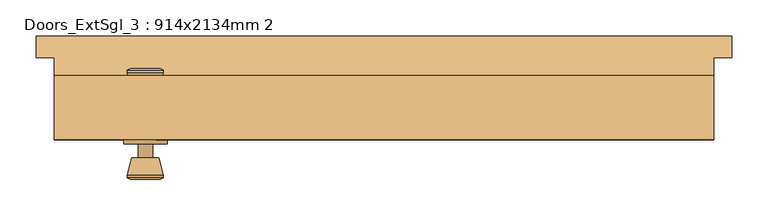
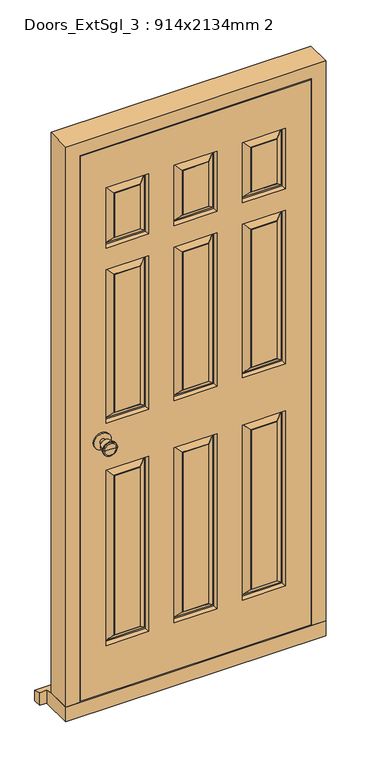
"""IFC4 building model written with IfcOpenShell, lengths in millimetres: door geometry, Doors_ExtSgl_3 : 914x2134mm 2."""

from ifc_helpers import new_model, si_unit, point, frame, frame_2d, origin, place, context, project, spatial, polyline, circle_curve, trimmed, segment, composite_curve, outline, extrude, faceted_brep, source, transform, mapped, element, save
from ifc_brep_helpers import plane_surface, cylinder_surface, revolved_surface, advanced_brep


def doors_extsgl_3_914x2134mm_2_3fd9b232(model_context):
    return source(origin(), model_context, "Body", "SolidModel", [
        advanced_brep(
        [(-330.6666667, -43.8, 1000.0), (-320.6666667, -43.8, 1000.0), (-340.6666667, -43.8, 1000.0), (-310.1907991, -92.8, 1000.0), (-330.6666667, -92.8, 1000.0), (-351.1425342, -92.8, 1000.0), (-305.6666667, -90.9721319, 1000.0), (-355.6666667, -90.9721319, 1000.0), (-305.6666667, -87.5084537, 1000.0), (-355.6666667, -87.5084537, 1000.0), (-312.0304306, -62.8, 1000.0), (-349.3029027, -62.8, 1000.0), (-320.6666667, -62.8, 1000.0), (-340.6666667, -62.8, 1000.0)],
        [
            (0, 1),
            (1, 2, circle_curve(frame((-330.6666667, -43.8, 1000.0), z_axis=(0.0, 1.0, 0.0), x_axis=(-1.0, 0.0, 0.0)), 10.0)),
            (2, 0),
            (2, 1, circle_curve(frame((-330.6666667, -43.8, 1000.0), z_axis=(0.0, 1.0, 0.0), x_axis=(-1.0, 0.0, 0.0)), 10.0)),
            (3, 4),
            (4, 5),
            (5, 3, circle_curve(frame((-330.6666667, -92.8, 1000.0), z_axis=(0.0, -1.0, 0.0), x_axis=(-1.0, 0.0, 0.0)), 20.4758676)),
            (3, 5, circle_curve(frame((-330.6666667, -92.8, 1000.0), z_axis=(0.0, -1.0, 0.0), x_axis=(-1.0, 0.0, 0.0)), 20.4758676)),
            (6, 3),
            (5, 7),
            (7, 6, circle_curve(frame((-330.6666667, -90.9721319, 1000.0), z_axis=(0.0, -1.0, 0.0), x_axis=(-1.0, 0.0, 0.0)), 25.0)),
            (6, 7, circle_curve(frame((-330.6666667, -90.9721319, 1000.0), z_axis=(0.0, -1.0, 0.0), x_axis=(-1.0, 0.0, 0.0)), 25.0)),
            (8, 6),
            (7, 9),
            (9, 8, circle_curve(frame((-330.6666667, -87.5084537, 1000.0), z_axis=(0.0, -1.0, 0.0), x_axis=(-1.0, 0.0, 0.0)), 25.0)),
            (8, 9, circle_curve(frame((-330.6666667, -87.5084537, 1000.0), z_axis=(0.0, -1.0, 0.0), x_axis=(-1.0, 0.0, 0.0)), 25.0)),
            (10, 8),
            (9, 11),
            (11, 10, circle_curve(frame((-330.6666667, -62.8, 1000.0), z_axis=(0.0, -1.0, 0.0), x_axis=(-1.0, 0.0, 0.0)), 18.636236)),
            (10, 11, circle_curve(frame((-330.6666667, -62.8, 1000.0), z_axis=(0.0, -1.0, 0.0), x_axis=(-1.0, 0.0, 0.0)), 18.636236)),
            (12, 10),
            (11, 13),
            (13, 12, circle_curve(frame((-330.6666667, -62.8, 1000.0), z_axis=(0.0, -1.0, 0.0), x_axis=(-1.0, 0.0, 0.0)), 10.0)),
            (12, 13, circle_curve(frame((-330.6666667, -62.8, 1000.0), z_axis=(0.0, -1.0, 0.0), x_axis=(-1.0, 0.0, 0.0)), 10.0)),
            (1, 12),
            (13, 2),
        ],
        [
            plane_surface(frame((-330.6666667, -43.8, 1000.0), z_axis=(0.0, 1.0, 0.0), x_axis=(-1.0, 0.0, 0.0))),
            plane_surface(frame((-330.6666667, -92.8, 1000.0), z_axis=(0.0, -1.0, 0.0), x_axis=(-1.0, 0.0, 0.0))),
            revolved_surface(polyline([(-351.1425342, -92.8, 1000.0), (-355.6666667, -90.9721319, 1000.0)]), (-330.6666667, -43.8, 1000.0), (0.0, 1.0, 0.0)),
            cylinder_surface(frame((-330.6666667, -43.8, 1000.0), z_axis=(0.0, 1.0, 0.0), x_axis=(-1.0, 0.0, 0.0)), 25.0),
            revolved_surface(polyline([(-355.6666667, -87.5084537, 1000.0), (-349.3029027, -62.8, 1000.0)]), (-330.6666667, -43.8, 1000.0), (0.0, 1.0, 0.0)),
            plane_surface(frame((-330.6666667, -62.8, 1000.0), z_axis=(0.0, 1.0, 0.0), x_axis=(-1.0, 0.0, 0.0))),
            cylinder_surface(frame((-330.6666667, -43.8, 1000.0), z_axis=(0.0, 1.0, 0.0), x_axis=(-1.0, 0.0, 0.0)), 10.0),
        ],
        [
            (0, [[1, 2, 3]]),
            (0, [[-3, 4, -1]]),
            (1, [[5, 6, 7]]),
            (1, [[-6, -5, 8]]),
            (2, [[9, -7, 10, 11]]),
            (2, [[-10, -8, -9, 12]]),
            (3, [[13, -11, 14, 15]]),
            (3, [[-14, -12, -13, 16]]),
            (4, [[17, -15, 18, 19]]),
            (4, [[-18, -16, -17, 20]]),
            (5, [[21, -19, 22, 23]]),
            (5, [[-22, -20, -21, 24]]),
            (6, [[25, -23, 26, -2]]),
            (6, [[-26, -24, -25, -4]]),
        ],
    ),
        extrude(outline(composite_curve([segment(trimmed(circle_curve(frame_2d((1000.0, -330.6666667)), 30.0), [point((1000.0, -360.6666667))], [point((1000.0, -300.6666667))], False, "CARTESIAN"), True, "CONTINUOUS"), segment(trimmed(circle_curve(frame_2d((1000.0, -330.6666667)), 30.0), [point((1000.0, -300.6666667))], [point((1000.0, -360.6666667))], False, "CARTESIAN"), True, "CONTINUOUS")], self_intersect=False)), frame((0.0, -43.8, 0.0), z_axis=(0.0, 1.0, 0.0), x_axis=(0.0, 0.0, 1.0)), (0.0, 0.0, 1.0), 6.0),
        advanced_brep(
        [(-330.6666667, 12.2, 1000.0), (-340.6666667, 12.2, 1000.0), (-320.6666667, 12.2, 1000.0), (-310.1907991, 61.2, 1000.0), (-351.1425342, 61.2, 1000.0), (-330.6666667, 61.2, 1000.0), (-305.6666667, 59.3721319, 1000.0), (-355.6666667, 59.3721319, 1000.0), (-305.6666667, 55.9084537, 1000.0), (-355.6666667, 55.9084537, 1000.0), (-312.0304306, 31.2, 1000.0), (-349.3029027, 31.2, 1000.0), (-320.6666667, 31.2, 1000.0), (-340.6666667, 31.2, 1000.0)],
        [
            (0, 1),
            (1, 2, circle_curve(frame((-330.6666667, 12.2, 1000.0), z_axis=(0.0, -1.0, 0.0), x_axis=(-1.0, 0.0, 0.0)), 10.0)),
            (2, 0),
            (2, 1, circle_curve(frame((-330.6666667, 12.2, 1000.0), z_axis=(0.0, -1.0, 0.0), x_axis=(-1.0, 0.0, 0.0)), 10.0)),
            (3, 4, circle_curve(frame((-330.6666667, 61.2, 1000.0), z_axis=(0.0, 1.0, 0.0), x_axis=(-1.0, 0.0, 0.0)), 20.4758676)),
            (4, 5),
            (5, 3),
            (4, 3, circle_curve(frame((-330.6666667, 61.2, 1000.0), z_axis=(0.0, 1.0, 0.0), x_axis=(-1.0, 0.0, 0.0)), 20.4758676)),
            (6, 7, circle_curve(frame((-330.6666667, 59.3721319, 1000.0), z_axis=(0.0, 1.0, 0.0), x_axis=(-1.0, 0.0, 0.0)), 25.0)),
            (7, 4),
            (3, 6),
            (7, 6, circle_curve(frame((-330.6666667, 59.3721319, 1000.0), z_axis=(0.0, 1.0, 0.0), x_axis=(-1.0, 0.0, 0.0)), 25.0)),
            (8, 9, circle_curve(frame((-330.6666667, 55.9084537, 1000.0), z_axis=(0.0, 1.0, 0.0), x_axis=(-1.0, 0.0, 0.0)), 25.0)),
            (9, 7),
            (6, 8),
            (9, 8, circle_curve(frame((-330.6666667, 55.9084537, 1000.0), z_axis=(0.0, 1.0, 0.0), x_axis=(-1.0, 0.0, 0.0)), 25.0)),
            (10, 11, circle_curve(frame((-330.6666667, 31.2, 1000.0), z_axis=(0.0, 1.0, 0.0), x_axis=(-1.0, 0.0, 0.0)), 18.636236)),
            (11, 9),
            (8, 10),
            (11, 10, circle_curve(frame((-330.6666667, 31.2, 1000.0), z_axis=(0.0, 1.0, 0.0), x_axis=(-1.0, 0.0, 0.0)), 18.636236)),
            (12, 13, circle_curve(frame((-330.6666667, 31.2, 1000.0), z_axis=(0.0, 1.0, 0.0), x_axis=(-1.0, 0.0, 0.0)), 10.0)),
            (13, 11),
            (10, 12),
            (13, 12, circle_curve(frame((-330.6666667, 31.2, 1000.0), z_axis=(0.0, 1.0, 0.0), x_axis=(-1.0, 0.0, 0.0)), 10.0)),
            (1, 13),
            (12, 2),
        ],
        [
            plane_surface(frame((-330.6666667, 12.2, 1000.0), z_axis=(0.0, -1.0, 0.0), x_axis=(-1.0, 0.0, 0.0))),
            plane_surface(frame((-330.6666667, 61.2, 1000.0), z_axis=(0.0, 1.0, 0.0), x_axis=(-1.0, 0.0, 0.0))),
            revolved_surface(polyline([(-351.1425342, 61.2, 1000.0), (-355.6666667, 59.3721319, 1000.0)]), (-330.6666667, 12.2, 1000.0), (0.0, -1.0, 0.0)),
            cylinder_surface(frame((-330.6666667, 12.2, 1000.0), z_axis=(0.0, -1.0, 0.0), x_axis=(-1.0, 0.0, 0.0)), 25.0),
            revolved_surface(polyline([(-355.6666667, 55.9084537, 1000.0), (-349.3029027, 31.2, 1000.0)]), (-330.6666667, 12.2, 1000.0), (0.0, -1.0, 0.0)),
            plane_surface(frame((-330.6666667, 31.2, 1000.0), z_axis=(0.0, -1.0, 0.0), x_axis=(-1.0, 0.0, 0.0))),
            cylinder_surface(frame((-330.6666667, 12.2, 1000.0), z_axis=(0.0, -1.0, 0.0), x_axis=(-1.0, 0.0, 0.0)), 10.0),
        ],
        [
            (0, [[1, 2, 3]]),
            (0, [[-3, 4, -1]]),
            (1, [[5, 6, 7]]),
            (1, [[8, -7, -6]]),
            (2, [[9, 10, -5, 11]]),
            (2, [[12, -11, -8, -10]]),
            (3, [[13, 14, -9, 15]]),
            (3, [[16, -15, -12, -14]]),
            (4, [[17, 18, -13, 19]]),
            (4, [[20, -19, -16, -18]]),
            (5, [[21, 22, -17, 23]]),
            (5, [[24, -23, -20, -22]]),
            (6, [[-2, 25, -21, 26]]),
            (6, [[-4, -26, -24, -25]]),
        ],
    ),
        extrude(outline(composite_curve([segment(trimmed(circle_curve(frame_2d((1000.0, -330.6666667)), 30.0), [point((1000.0, -360.6666667))], [point((1000.0, -300.6666667))], False, "CARTESIAN"), True, "CONTINUOUS"), segment(trimmed(circle_curve(frame_2d((1000.0, -330.6666667)), 30.0), [point((1000.0, -300.6666667))], [point((1000.0, -360.6666667))], False, "CARTESIAN"), True, "CONTINUOUS")], self_intersect=False)), frame((0.0, 6.2, 0.0), z_axis=(0.0, 1.0, 0.0), x_axis=(0.0, 0.0, 1.0)), (0.0, 0.0, 1.0), 6.0),
        faceted_brep([(386.7333333, 51.2, 54.5), (457.2333333, 51.2, 54.5), (457.2333333, -37.8, 54.5), (408.7333333, -37.8, 54.5), (408.7333333, 9.2, 54.5), (386.7333333, 9.2, 54.5), (386.7333333, 51.2, 2063.1), (-386.6666667, 51.2, 2063.1), (-386.6666667, 51.2, 54.5), (-457.1666667, 51.2, 54.5), (-457.1666667, 51.2, 2133.6), (457.2333333, 51.2, 2133.6), (457.2333333, -37.8, 2133.6), (-457.1666667, -37.8, 2133.6), (-457.1666667, -37.8, 54.5), (-408.6666667, -37.8, 54.5), (-408.6666667, -37.8, 2085.1), (408.7333333, -37.8, 2085.1), (408.7333333, 9.2, 2085.1), (-408.6666667, 9.2, 2085.1), (-408.6666667, 9.2, 54.5), (-386.6666667, 9.2, 54.5), (-386.6666667, 9.2, 2063.1), (386.7333333, 9.2, 2063.1)], [[[0, 1, 2, 3, 4, 5]], [[1, 0, 6, 7, 8, 9, 10, 11]], [[2, 1, 11, 12]], [[3, 2, 12, 13, 14, 15, 16, 17]], [[4, 3, 17, 18]], [[5, 4, 18, 19, 20, 21, 22, 23]], [[0, 5, 23, 6]], [[8, 7, 22, 21]], [[9, 8, 21, 20, 15, 14]], [[10, 9, 14, 13]], [[16, 15, 20, 19]], [[11, 10, 13, 12]], [[17, 16, 19, 18]], [[7, 6, 23, 22]]]),
        faceted_brep([(405.7333333, -37.8, 58.5), (405.7333333, -37.8, 2082.1), (-406.5916961, -37.8, 2082.1), (-406.5916961, -37.8, 58.5), (-165.2, -37.8, 883.5), (-165.2, -37.8, 233.5), (-315.6666667, -37.8, 233.5), (-315.6666667, -37.8, 883.5), (315.7333333, -37.8, 883.5), (315.7333333, -37.8, 233.5), (165.2666667, -37.8, 233.5), (165.2666667, -37.8, 883.5), (75.2666667, -37.8, 883.5), (75.2666667, -37.8, 233.5), (-75.2, -37.8, 233.5), (-75.2, -37.8, 883.5), (-315.6666667, -37.8, 1058.5), (-315.6666667, -37.8, 1628.5), (-165.2, -37.8, 1628.5), (-165.2, -37.8, 1058.5), (75.2666667, -37.8, 1628.5), (75.2666667, -37.8, 1058.5), (-75.2, -37.8, 1058.5), (-75.2, -37.8, 1628.5), (315.7333333, -37.8, 1628.5), (315.7333333, -37.8, 1058.5), (165.2666667, -37.8, 1058.5), (165.2666667, -37.8, 1628.5), (-165.2, -37.8, 1932.1), (-165.2, -37.8, 1708.5), (-315.6666667, -37.8, 1708.5), (-315.6666667, -37.8, 1932.1), (75.2666667, -37.8, 1932.1), (75.2666667, -37.8, 1708.5), (-75.2, -37.8, 1708.5), (-75.2, -37.8, 1932.1), (315.7333333, -37.8, 1932.1), (315.7333333, -37.8, 1708.5), (165.2666667, -37.8, 1708.5), (165.2666667, -37.8, 1932.1), (-195.2, -37.8, 263.5), (-195.2, -37.8, 853.5), (-285.6666667, -37.8, 853.5), (-285.6666667, -37.8, 263.5), (285.7333333, -37.8, 263.5), (285.7333333, -37.8, 853.5), (195.2666667, -37.8, 853.5), (195.2666667, -37.8, 263.5), (45.2666667, -37.8, 263.5), (45.2666667, -37.8, 853.5), (-45.2, -37.8, 853.5), (-45.2, -37.8, 263.5), (-285.6666667, -37.8, 1598.5), (-285.6666667, -37.8, 1088.5), (-195.2, -37.8, 1088.5), (-195.2, -37.8, 1598.5), (45.2666667, -37.8, 1088.5), (45.2666667, -37.8, 1598.5), (-45.2, -37.8, 1598.5), (-45.2, -37.8, 1088.5), (285.7333333, -37.8, 1088.5), (285.7333333, -37.8, 1598.5), (195.2666667, -37.8, 1598.5), (195.2666667, -37.8, 1088.5), (-195.2, -37.8, 1738.5), (-195.2, -37.8, 1902.1), (-285.6666667, -37.8, 1902.1), (-285.6666667, -37.8, 1738.5), (45.2666667, -37.8, 1738.5), (45.2666667, -37.8, 1902.1), (-45.2, -37.8, 1902.1), (-45.2, -37.8, 1738.5), (285.7333333, -37.8, 1738.5), (285.7333333, -37.8, 1902.1), (195.2666667, -37.8, 1902.1), (195.2666667, -37.8, 1738.5), (405.7333333, 6.2, 58.5), (-406.5916961, 6.2, 58.5), (-406.5916961, 6.2, 2082.1), (405.7333333, 6.2, 2082.1), (165.2666667, 6.2, 883.5), (165.2666667, 6.2, 233.5), (315.7333333, 6.2, 233.5), (315.7333333, 6.2, 883.5), (-315.6666667, 6.2, 883.5), (-315.6666667, 6.2, 233.5), (-165.2, 6.2, 233.5), (-165.2, 6.2, 883.5), (-75.2, 6.2, 883.5), (-75.2, 6.2, 233.5), (75.2666667, 6.2, 233.5), (75.2666667, 6.2, 883.5), (165.2666667, 6.2, 1628.5), (165.2666667, 6.2, 1058.5), (315.7333333, 6.2, 1058.5), (315.7333333, 6.2, 1628.5), (-75.2, 6.2, 1628.5), (-75.2, 6.2, 1058.5), (75.2666667, 6.2, 1058.5), (75.2666667, 6.2, 1628.5), (-315.6666667, 6.2, 1628.5), (-315.6666667, 6.2, 1058.5), (-165.2, 6.2, 1058.5), (-165.2, 6.2, 1628.5), (315.7333333, 6.2, 1708.5), (315.7333333, 6.2, 1932.1), (165.2666667, 6.2, 1932.1), (165.2666667, 6.2, 1708.5), (-75.2, 6.2, 1932.1), (-75.2, 6.2, 1708.5), (75.2666667, 6.2, 1708.5), (75.2666667, 6.2, 1932.1), (-315.6666667, 6.2, 1932.1), (-315.6666667, 6.2, 1708.5), (-165.2, 6.2, 1708.5), (-165.2, 6.2, 1932.1), (195.2666667, 6.2, 263.5), (195.2666667, 6.2, 853.5), (285.7333333, 6.2, 853.5), (285.7333333, 6.2, 263.5), (-285.6666667, 6.2, 263.5), (-285.6666667, 6.2, 853.5), (-195.2, 6.2, 853.5), (-195.2, 6.2, 263.5), (-45.2, 6.2, 263.5), (-45.2, 6.2, 853.5), (45.2666667, 6.2, 853.5), (45.2666667, 6.2, 263.5), (195.2666667, 6.2, 1088.5), (195.2666667, 6.2, 1598.5), (285.7333333, 6.2, 1598.5), (285.7333333, 6.2, 1088.5), (-45.2, 6.2, 1088.5), (-45.2, 6.2, 1598.5), (45.2666667, 6.2, 1598.5), (45.2666667, 6.2, 1088.5), (-285.6666667, 6.2, 1088.5), (-285.6666667, 6.2, 1598.5), (-195.2, 6.2, 1598.5), (-195.2, 6.2, 1088.5), (285.7333333, 6.2, 1902.1), (285.7333333, 6.2, 1738.5), (195.2666667, 6.2, 1738.5), (195.2666667, 6.2, 1902.1), (-45.2, 6.2, 1738.5), (-45.2, 6.2, 1902.1), (45.2666667, 6.2, 1902.1), (45.2666667, 6.2, 1738.5), (-285.6666667, 6.2, 1738.5), (-285.6666667, 6.2, 1902.1), (-195.2, 6.2, 1902.1), (-195.2, 6.2, 1738.5), (168.2666667, -8.8, 880.5), (168.2666667, -8.8, 236.5), (193.2666667, 5.2, 855.5), (193.2666667, 5.2, 261.5), (173.2666667, -8.8, 241.5), (173.2666667, -8.8, 875.5), (195.2666667, 5.2, 263.5), (195.2666667, 5.2, 853.5), (312.7333333, -8.8, 236.5), (287.7333333, 5.2, 261.5), (307.7333333, -8.8, 241.5), (285.7333333, 5.2, 263.5), (312.7333333, -8.8, 880.5), (287.7333333, 5.2, 855.5), (307.7333333, -8.8, 875.5), (285.7333333, 5.2, 853.5), (-312.6666667, -8.8, 880.5), (-312.6666667, -8.8, 236.5), (-287.6666667, 5.2, 855.5), (-287.6666667, 5.2, 261.5), (-307.6666667, -8.8, 241.5), (-307.6666667, -8.8, 875.5), (-285.6666667, 5.2, 263.5), (-285.6666667, 5.2, 853.5), (-168.2, -8.8, 236.5), (-193.2, 5.2, 261.5), (-173.2, -8.8, 241.5), (-195.2, 5.2, 263.5), (-168.2, -8.8, 880.5), (-193.2, 5.2, 855.5), (-173.2, -8.8, 875.5), (-195.2, 5.2, 853.5), (-195.2, -36.8, 263.5), (-195.2, -36.8, 853.5), (-173.2, -22.8, 241.5), (-173.2, -22.8, 875.5), (-193.2, -36.8, 855.5), (-193.2, -36.8, 261.5), (-168.2, -22.8, 880.5), (-168.2, -22.8, 236.5), (-285.6666667, -36.8, 853.5), (-307.6666667, -22.8, 875.5), (-287.6666667, -36.8, 855.5), (-312.6666667, -22.8, 880.5), (-285.6666667, -36.8, 263.5), (-307.6666667, -22.8, 241.5), (-287.6666667, -36.8, 261.5), (-312.6666667, -22.8, 236.5), (312.7333333, -22.8, 880.5), (312.7333333, -22.8, 236.5), (287.7333333, -36.8, 855.5), (287.7333333, -36.8, 261.5), (307.7333333, -22.8, 241.5), (307.7333333, -22.8, 875.5), (285.7333333, -36.8, 263.5), (285.7333333, -36.8, 853.5), (168.2666667, -22.8, 236.5), (193.2666667, -36.8, 261.5), (173.2666667, -22.8, 241.5), (195.2666667, -36.8, 263.5), (168.2666667, -22.8, 880.5), (193.2666667, -36.8, 855.5), (173.2666667, -22.8, 875.5), (195.2666667, -36.8, 853.5), (-45.2, 5.2, 263.5), (-45.2, 5.2, 853.5), (-67.2, -8.8, 241.5), (-67.2, -8.8, 875.5), (-47.2, 5.2, 855.5), (-47.2, 5.2, 261.5), (-72.2, -8.8, 880.5), (-72.2, -8.8, 236.5), (45.2666667, 5.2, 853.5), (67.2666667, -8.8, 875.5), (47.2666667, 5.2, 855.5), (72.2666667, -8.8, 880.5), (45.2666667, 5.2, 263.5), (67.2666667, -8.8, 241.5), (47.2666667, 5.2, 261.5), (72.2666667, -8.8, 236.5), (72.2666667, -22.8, 880.5), (72.2666667, -22.8, 236.5), (47.2666667, -36.8, 855.5), (47.2666667, -36.8, 261.5), (67.2666667, -22.8, 241.5), (67.2666667, -22.8, 875.5), (45.2666667, -36.8, 263.5), (45.2666667, -36.8, 853.5), (-72.2, -22.8, 236.5), (-47.2, -36.8, 261.5), (-67.2, -22.8, 241.5), (-45.2, -36.8, 263.5), (-72.2, -22.8, 880.5), (-47.2, -36.8, 855.5), (-67.2, -22.8, 875.5), (-45.2, -36.8, 853.5), (195.2666667, 5.2, 1088.5), (195.2666667, 5.2, 1598.5), (173.2666667, -8.8, 1066.5), (173.2666667, -8.8, 1620.5), (193.2666667, 5.2, 1600.5), (193.2666667, 5.2, 1086.5), (168.2666667, -8.8, 1625.5), (168.2666667, -8.8, 1061.5), (285.7333333, 5.2, 1598.5), (307.7333333, -8.8, 1620.5), (287.7333333, 5.2, 1600.5), (312.7333333, -8.8, 1625.5), (285.7333333, 5.2, 1088.5), (307.7333333, -8.8, 1066.5), (287.7333333, 5.2, 1086.5), (312.7333333, -8.8, 1061.5), (-45.2, 5.2, 1088.5), (-45.2, 5.2, 1598.5), (-67.2, -8.8, 1066.5), (-67.2, -8.8, 1620.5), (-47.2, 5.2, 1600.5), (-47.2, 5.2, 1086.5), (-72.2, -8.8, 1625.5), (-72.2, -8.8, 1061.5), (45.2666667, 5.2, 1598.5), (67.2666667, -8.8, 1620.5), (47.2666667, 5.2, 1600.5), (72.2666667, -8.8, 1625.5), (45.2666667, 5.2, 1088.5), (67.2666667, -8.8, 1066.5), (47.2666667, 5.2, 1086.5), (72.2666667, -8.8, 1061.5), (-285.6666667, 5.2, 1088.5), (-285.6666667, 5.2, 1598.5), (-307.6666667, -8.8, 1066.5), (-307.6666667, -8.8, 1620.5), (-287.6666667, 5.2, 1600.5), (-287.6666667, 5.2, 1086.5), (-312.6666667, -8.8, 1625.5), (-312.6666667, -8.8, 1061.5), (-195.2, 5.2, 1598.5), (-173.2, -8.8, 1620.5), (-193.2, 5.2, 1600.5), (-168.2, -8.8, 1625.5), (-195.2, 5.2, 1088.5), (-173.2, -8.8, 1066.5), (-193.2, 5.2, 1086.5), (-168.2, -8.8, 1061.5), (285.7333333, 5.2, 1902.1), (285.7333333, 5.2, 1738.5), (307.7333333, -8.8, 1924.1), (307.7333333, -8.8, 1716.5), (287.7333333, 5.2, 1736.5), (287.7333333, 5.2, 1904.1), (312.7333333, -8.8, 1711.5), (312.7333333, -8.8, 1929.1), (195.2666667, 5.2, 1738.5), (173.2666667, -8.8, 1716.5), (193.2666667, 5.2, 1736.5), (168.2666667, -8.8, 1711.5), (195.2666667, 5.2, 1902.1), (173.2666667, -8.8, 1924.1), (193.2666667, 5.2, 1904.1), (168.2666667, -8.8, 1929.1), (-45.2, 5.2, 1738.5), (-45.2, 5.2, 1902.1), (-67.2, -8.8, 1716.5), (-67.2, -8.8, 1924.1), (-47.2, 5.2, 1904.1), (-47.2, 5.2, 1736.5), (-72.2, -8.8, 1929.1), (-72.2, -8.8, 1711.5), (45.2666667, 5.2, 1902.1), (67.2666667, -8.8, 1924.1), (47.2666667, 5.2, 1904.1), (72.2666667, -8.8, 1929.1), (45.2666667, 5.2, 1738.5), (67.2666667, -8.8, 1716.5), (47.2666667, 5.2, 1736.5), (72.2666667, -8.8, 1711.5), (-285.6666667, 5.2, 1738.5), (-285.6666667, 5.2, 1902.1), (-307.6666667, -8.8, 1716.5), (-307.6666667, -8.8, 1924.1), (-287.6666667, 5.2, 1904.1), (-287.6666667, 5.2, 1736.5), (-312.6666667, -8.8, 1929.1), (-312.6666667, -8.8, 1711.5), (-195.2, 5.2, 1902.1), (-173.2, -8.8, 1924.1), (-193.2, 5.2, 1904.1), (-168.2, -8.8, 1929.1), (-195.2, 5.2, 1738.5), (-173.2, -8.8, 1716.5), (-193.2, 5.2, 1736.5), (-168.2, -8.8, 1711.5), (-312.6666667, -22.8, 1061.5), (-312.6666667, -22.8, 1625.5), (-287.6666667, -36.8, 1086.5), (-287.6666667, -36.8, 1600.5), (-307.6666667, -22.8, 1620.5), (-307.6666667, -22.8, 1066.5), (-285.6666667, -36.8, 1598.5), (-285.6666667, -36.8, 1088.5), (-168.2, -22.8, 1625.5), (-193.2, -36.8, 1600.5), (-173.2, -22.8, 1620.5), (-195.2, -36.8, 1598.5), (-168.2, -22.8, 1061.5), (-193.2, -36.8, 1086.5), (-173.2, -22.8, 1066.5), (-195.2, -36.8, 1088.5), (45.2666667, -36.8, 1088.5), (45.2666667, -36.8, 1598.5), (67.2666667, -22.8, 1066.5), (67.2666667, -22.8, 1620.5), (47.2666667, -36.8, 1600.5), (47.2666667, -36.8, 1086.5), (72.2666667, -22.8, 1625.5), (72.2666667, -22.8, 1061.5), (-45.2, -36.8, 1598.5), (-67.2, -22.8, 1620.5), (-47.2, -36.8, 1600.5), (-72.2, -22.8, 1625.5), (-45.2, -36.8, 1088.5), (-67.2, -22.8, 1066.5), (-47.2, -36.8, 1086.5), (-72.2, -22.8, 1061.5), (312.7333333, -22.8, 1625.5), (312.7333333, -22.8, 1061.5), (287.7333333, -36.8, 1600.5), (287.7333333, -36.8, 1086.5), (307.7333333, -22.8, 1066.5), (307.7333333, -22.8, 1620.5), (285.7333333, -36.8, 1088.5), (285.7333333, -36.8, 1598.5), (168.2666667, -22.8, 1061.5), (193.2666667, -36.8, 1086.5), (173.2666667, -22.8, 1066.5), (195.2666667, -36.8, 1088.5), (168.2666667, -22.8, 1625.5), (193.2666667, -36.8, 1600.5), (173.2666667, -22.8, 1620.5), (195.2666667, -36.8, 1598.5), (-195.2, -36.8, 1738.5), (-195.2, -36.8, 1902.1), (-173.2, -22.8, 1716.5), (-173.2, -22.8, 1924.1), (-193.2, -36.8, 1904.1), (-193.2, -36.8, 1736.5), (-168.2, -22.8, 1929.1), (-168.2, -22.8, 1711.5), (-285.6666667, -36.8, 1902.1), (-307.6666667, -22.8, 1924.1), (-287.6666667, -36.8, 1904.1), (-312.6666667, -22.8, 1929.1), (-285.6666667, -36.8, 1738.5), (-307.6666667, -22.8, 1716.5), (-287.6666667, -36.8, 1736.5), (-312.6666667, -22.8, 1711.5), (45.2666667, -36.8, 1738.5), (45.2666667, -36.8, 1902.1), (67.2666667, -22.8, 1716.5), (67.2666667, -22.8, 1924.1), (47.2666667, -36.8, 1904.1), (47.2666667, -36.8, 1736.5), (72.2666667, -22.8, 1929.1), (72.2666667, -22.8, 1711.5), (-45.2, -36.8, 1902.1), (-67.2, -22.8, 1924.1), (-47.2, -36.8, 1904.1), (-72.2, -22.8, 1929.1), (-45.2, -36.8, 1738.5), (-67.2, -22.8, 1716.5), (-47.2, -36.8, 1736.5), (-72.2, -22.8, 1711.5), (285.7333333, -36.8, 1738.5), (285.7333333, -36.8, 1902.1), (307.7333333, -22.8, 1716.5), (307.7333333, -22.8, 1924.1), (287.7333333, -36.8, 1904.1), (287.7333333, -36.8, 1736.5), (312.7333333, -22.8, 1929.1), (312.7333333, -22.8, 1711.5), (195.2666667, -36.8, 1902.1), (173.2666667, -22.8, 1924.1), (193.2666667, -36.8, 1904.1), (168.2666667, -22.8, 1929.1), (195.2666667, -36.8, 1738.5), (173.2666667, -22.8, 1716.5), (193.2666667, -36.8, 1736.5), (168.2666667, -22.8, 1711.5)], [[[0, 1, 2, 3], [4, 5, 6, 7], [8, 9, 10, 11], [12, 13, 14, 15], [16, 17, 18, 19], [20, 21, 22, 23], [24, 25, 26, 27], [28, 29, 30, 31], [32, 33, 34, 35], [36, 37, 38, 39]], [[40, 41, 42, 43]], [[44, 45, 46, 47]], [[48, 49, 50, 51]], [[52, 53, 54, 55]], [[56, 57, 58, 59]], [[60, 61, 62, 63]], [[64, 65, 66, 67]], [[68, 69, 70, 71]], [[72, 73, 74, 75]], [[76, 77, 78, 79], [80, 81, 82, 83], [84, 85, 86, 87], [88, 89, 90, 91], [92, 93, 94, 95], [96, 97, 98, 99], [100, 101, 102, 103], [104, 105, 106, 107], [108, 109, 110, 111], [112, 113, 114, 115]], [[116, 117, 118, 119]], [[120, 121, 122, 123]], [[124, 125, 126, 127]], [[128, 129, 130, 131]], [[132, 133, 134, 135]], [[136, 137, 138, 139]], [[140, 141, 142, 143]], [[144, 145, 146, 147]], [[148, 149, 150, 151]], [[1, 0, 76, 79]], [[2, 1, 79, 78]], [[3, 2, 78, 77]], [[0, 3, 77, 76]], [[152, 153, 81, 80]], [[154, 155, 156, 157]], [[116, 158, 159, 117]], [[81, 153, 160, 82]], [[156, 155, 161, 162]], [[158, 116, 119, 163]], [[82, 160, 164, 83]], [[162, 161, 165, 166]], [[163, 119, 118, 167]], [[152, 80, 83, 164]], [[153, 152, 164, 160], [157, 156, 162, 166]], [[154, 157, 166, 165]], [[155, 154, 165, 161], [159, 158, 163, 167]], [[117, 159, 167, 118]], [[168, 169, 85, 84]], [[170, 171, 172, 173]], [[120, 174, 175, 121]], [[85, 169, 176, 86]], [[172, 171, 177, 178]], [[174, 120, 123, 179]], [[86, 176, 180, 87]], [[178, 177, 181, 182]], [[179, 123, 122, 183]], [[168, 84, 87, 180]], [[169, 168, 180, 176], [173, 172, 178, 182]], [[170, 173, 182, 181]], [[171, 170, 181, 177], [175, 174, 179, 183]], [[121, 175, 183, 122]], [[184, 185, 41, 40]], [[186, 187, 188, 189]], [[4, 190, 191, 5]], [[41, 185, 192, 42]], [[188, 187, 193, 194]], [[190, 4, 7, 195]], [[42, 192, 196, 43]], [[194, 193, 197, 198]], [[195, 7, 6, 199]], [[184, 40, 43, 196]], [[189, 188, 194, 198], [185, 184, 196, 192]], [[186, 189, 198, 197]], [[191, 190, 195, 199], [187, 186, 197, 193]], [[5, 191, 199, 6]], [[200, 201, 9, 8]], [[202, 203, 204, 205]], [[44, 206, 207, 45]], [[9, 201, 208, 10]], [[204, 203, 209, 210]], [[206, 44, 47, 211]], [[10, 208, 212, 11]], [[210, 209, 213, 214]], [[211, 47, 46, 215]], [[200, 8, 11, 212]], [[201, 200, 212, 208], [205, 204, 210, 214]], [[202, 205, 214, 213]], [[203, 202, 213, 209], [207, 206, 211, 215]], [[45, 207, 215, 46]], [[216, 217, 125, 124]], [[218, 219, 220, 221]], [[88, 222, 223, 89]], [[125, 217, 224, 126]], [[220, 219, 225, 226]], [[222, 88, 91, 227]], [[126, 224, 228, 127]], [[226, 225, 229, 230]], [[227, 91, 90, 231]], [[216, 124, 127, 228]], [[221, 220, 226, 230], [217, 216, 228, 224]], [[218, 221, 230, 229]], [[223, 222, 227, 231], [219, 218, 229, 225]], [[89, 223, 231, 90]], [[232, 233, 13, 12]], [[234, 235, 236, 237]], [[48, 238, 239, 49]], [[13, 233, 240, 14]], [[236, 235, 241, 242]], [[238, 48, 51, 243]], [[14, 240, 244, 15]], [[242, 241, 245, 246]], [[243, 51, 50, 247]], [[232, 12, 15, 244]], [[233, 232, 244, 240], [237, 236, 242, 246]], [[234, 237, 246, 245]], [[235, 234, 245, 241], [239, 238, 243, 247]], [[49, 239, 247, 50]], [[248, 249, 129, 128]], [[250, 251, 252, 253]], [[92, 254, 255, 93]], [[129, 249, 256, 130]], [[252, 251, 257, 258]], [[254, 92, 95, 259]], [[130, 256, 260, 131]], [[258, 257, 261, 262]], [[259, 95, 94, 263]], [[248, 128, 131, 260]], [[253, 252, 258, 262], [249, 248, 260, 256]], [[250, 253, 262, 261]], [[255, 254, 259, 263], [251, 250, 261, 257]], [[93, 255, 263, 94]], [[264, 265, 133, 132]], [[266, 267, 268, 269]], [[96, 270, 271, 97]], [[133, 265, 272, 134]], [[268, 267, 273, 274]], [[270, 96, 99, 275]], [[134, 272, 276, 135]], [[274, 273, 277, 278]], [[275, 99, 98, 279]], [[264, 132, 135, 276]], [[269, 268, 274, 278], [265, 264, 276, 272]], [[266, 269, 278, 277]], [[271, 270, 275, 279], [267, 266, 277, 273]], [[97, 271, 279, 98]], [[280, 281, 137, 136]], [[282, 283, 284, 285]], [[100, 286, 287, 101]], [[137, 281, 288, 138]], [[284, 283, 289, 290]], [[286, 100, 103, 291]], [[138, 288, 292, 139]], [[290, 289, 293, 294]], [[291, 103, 102, 295]], [[280, 136, 139, 292]], [[285, 284, 290, 294], [281, 280, 292, 288]], [[282, 285, 294, 293]], [[287, 286, 291, 295], [283, 282, 293, 289]], [[101, 287, 295, 102]], [[296, 297, 141, 140]], [[298, 299, 300, 301]], [[104, 302, 303, 105]], [[141, 297, 304, 142]], [[300, 299, 305, 306]], [[302, 104, 107, 307]], [[142, 304, 308, 143]], [[306, 305, 309, 310]], [[307, 107, 106, 311]], [[296, 140, 143, 308]], [[301, 300, 306, 310], [297, 296, 308, 304]], [[298, 301, 310, 309]], [[303, 302, 307, 311], [299, 298, 309, 305]], [[105, 303, 311, 106]], [[312, 313, 145, 144]], [[314, 315, 316, 317]], [[108, 318, 319, 109]], [[145, 313, 320, 146]], [[316, 315, 321, 322]], [[318, 108, 111, 323]], [[146, 320, 324, 147]], [[322, 321, 325, 326]], [[323, 111, 110, 327]], [[312, 144, 147, 324]], [[317, 316, 322, 326], [313, 312, 324, 320]], [[314, 317, 326, 325]], [[319, 318, 323, 327], [315, 314, 325, 321]], [[109, 319, 327, 110]], [[328, 329, 149, 148]], [[330, 331, 332, 333]], [[112, 334, 335, 113]], [[149, 329, 336, 150]], [[332, 331, 337, 338]], [[334, 112, 115, 339]], [[150, 336, 340, 151]], [[338, 337, 341, 342]], [[339, 115, 114, 343]], [[328, 148, 151, 340]], [[333, 332, 338, 342], [329, 328, 340, 336]], [[330, 333, 342, 341]], [[335, 334, 339, 343], [331, 330, 341, 337]], [[113, 335, 343, 114]], [[344, 345, 17, 16]], [[346, 347, 348, 349]], [[52, 350, 351, 53]], [[17, 345, 352, 18]], [[348, 347, 353, 354]], [[350, 52, 55, 355]], [[18, 352, 356, 19]], [[354, 353, 357, 358]], [[355, 55, 54, 359]], [[344, 16, 19, 356]], [[345, 344, 356, 352], [349, 348, 354, 358]], [[346, 349, 358, 357]], [[347, 346, 357, 353], [351, 350, 355, 359]], [[53, 351, 359, 54]], [[360, 361, 57, 56]], [[362, 363, 364, 365]], [[20, 366, 367, 21]], [[57, 361, 368, 58]], [[364, 363, 369, 370]], [[366, 20, 23, 371]], [[58, 368, 372, 59]], [[370, 369, 373, 374]], [[371, 23, 22, 375]], [[360, 56, 59, 372]], [[365, 364, 370, 374], [361, 360, 372, 368]], [[362, 365, 374, 373]], [[367, 366, 371, 375], [363, 362, 373, 369]], [[21, 367, 375, 22]], [[376, 377, 25, 24]], [[378, 379, 380, 381]], [[60, 382, 383, 61]], [[25, 377, 384, 26]], [[380, 379, 385, 386]], [[382, 60, 63, 387]], [[26, 384, 388, 27]], [[386, 385, 389, 390]], [[387, 63, 62, 391]], [[376, 24, 27, 388]], [[377, 376, 388, 384], [381, 380, 386, 390]], [[378, 381, 390, 389]], [[379, 378, 389, 385], [383, 382, 387, 391]], [[61, 383, 391, 62]], [[392, 393, 65, 64]], [[394, 395, 396, 397]], [[28, 398, 399, 29]], [[65, 393, 400, 66]], [[396, 395, 401, 402]], [[398, 28, 31, 403]], [[66, 400, 404, 67]], [[402, 401, 405, 406]], [[403, 31, 30, 407]], [[392, 64, 67, 404]], [[397, 396, 402, 406], [393, 392, 404, 400]], [[394, 397, 406, 405]], [[399, 398, 403, 407], [395, 394, 405, 401]], [[29, 399, 407, 30]], [[408, 409, 69, 68]], [[410, 411, 412, 413]], [[32, 414, 415, 33]], [[69, 409, 416, 70]], [[412, 411, 417, 418]], [[414, 32, 35, 419]], [[70, 416, 420, 71]], [[418, 417, 421, 422]], [[419, 35, 34, 423]], [[408, 68, 71, 420]], [[413, 412, 418, 422], [409, 408, 420, 416]], [[410, 413, 422, 421]], [[415, 414, 419, 423], [411, 410, 421, 417]], [[33, 415, 423, 34]], [[424, 425, 73, 72]], [[426, 427, 428, 429]], [[36, 430, 431, 37]], [[73, 425, 432, 74]], [[428, 427, 433, 434]], [[430, 36, 39, 435]], [[74, 432, 436, 75]], [[434, 433, 437, 438]], [[435, 39, 38, 439]], [[424, 72, 75, 436]], [[429, 428, 434, 438], [425, 424, 436, 432]], [[426, 429, 438, 437]], [[431, 430, 435, 439], [427, 426, 437, 433]], [[37, 431, 439, 38]]]),
        faceted_brep([(482.2333333, 106.2, 0.0), (482.2333333, 106.2, 38.5947221), (482.2333333, 76.2, 47.2703282), (482.2333333, 76.2, 0.0), (-482.1666667, 106.2, 38.5947221), (-482.1666667, 106.2, 0.0), (-482.1666667, 76.2, 0.0), (-482.1666667, 76.2, 47.2703282), (457.2333333, 76.2, 0.0), (457.2333333, -37.8, 0.0), (-457.1666667, -37.8, 0.0), (-457.1666667, 76.2, 0.0), (-457.1666667, 76.2, 47.2703282), (-457.1666667, 51.2, 54.5), (457.2333333, 51.2, 54.5), (457.2333333, 76.2, 47.2703282), (-457.1666667, -37.8, 54.5), (457.2333333, -37.8, 54.5)], [[[0, 1, 2, 3]], [[4, 5, 6, 7]], [[5, 0, 3, 8, 9, 10, 11, 6]], [[1, 0, 5, 4]], [[1, 4, 7, 12, 13, 14, 15, 2]], [[13, 16, 17, 14]], [[16, 10, 9, 17]], [[12, 11, 10, 16, 13]], [[11, 12, 7, 6]], [[8, 15, 14, 17, 9]], [[15, 8, 3, 2]]]),
    ])


if __name__ == "__main__":
    model = new_model("IFC4")
    model_context = context("Model", 3, world=origin())
    ifc_project = project(units=[si_unit("LENGTHUNIT", "METRE", prefix="MILLI")], contexts=[model_context])
    site = spatial("IfcSite", under=ifc_project)
    building = spatial("IfcBuilding", under=site)
    placement = place(None, origin())
    doors_extsgl_3_914x2134mm_2_shape = doors_extsgl_3_914x2134mm_2_3fd9b232(model_context)
    element("IfcDoor", 1, ObjectType="Doors_ExtSgl_3 : 914x2134mm 2", at=placement, inside=building, context=model_context, shape_type="MappedRepresentation", body=[
        mapped(doors_extsgl_3_914x2134mm_2_shape, transform((0.0, 0.0, 0.0), x_axis=(1.0, 0.0, 0.0), y_axis=(0.0, 1.0, 0.0), z_axis=(0.0, 0.0, 1.0))),
    ])
    save(model, "model.ifc")

# Revit data of these elements
# Type "Doors_ExtSgl_3 : 914x2134mm 2"
#   Type Mark = "13"
#   Type Comments = "External Single"
#   Operation = "SingleSwingRight"
#   Construction Type Id = "MDOOR"
#   Keynote = "L20"
#   Analytic Construction = "Metal"
#   Wrap Layers (Int) from Ext = 0' - 6.98819"
#   Wrap Layers (Ext) from Ext = 0' - 4.03543"
#   Thickness = 0' - 1.73228"
#   Stile Top of Lock rail = 3' - 3.37008"
#   Stile Top of Frieze Rail = 5' - 4.96063"
#   Stile Top Rail = 0' - 5.90551"
#   Stile Shutting = 0' - 3.54331"
#   Stile Muntin Rail = 0' - 3.54331"
#   Stile Lock Rail = 0' - 6.88976"
#   Stile Intermediate/Frieze = 0' - 3.14961"
#   Stile Hanging = 0' - 3.54331"
#   Stile Bottom Rail = 0' - 6.88976"
#   Rough Width = 3' - 0"
#   Rough Height = 7' - 0"
#   O/A Frame Width = 0' - 2.51969"
#   Heat Transfer Coefficient (U) = 0.651978 BTU/(h·ft²·°F)
#   Handle Z Distance = 3' - 3.37008"
#   Glazing Thickness = 0' - 0.94488"
#   FrameWidth = 0' - 1.65354"
#   FrameOffset - External = 0' - 0.98425"
#   FrameDepth = 0' - 3.50394"
#   Door Panel Width = 2' - 7.94488"
#   Door Panel Thickness = 0' - 1.73228"
#   Door Panel Height = 6' - 7.66929"
#   DONT CHANGE - Panel Width = 0' - 5.92388"
#   Cill Thickness = 0' - 2.14567"
#   Cill Projection = 0' - 1.1811"
#   Handle X Distance = 0' - 2.95276"
#   Height = 7' - 0"
#   Structural Tolerance = 0' - 0.25591"
#   Tolerance = 0' - 0.11811"
#   Undercut = 0' - 0.15748"
#   Width = 3' - 0"
#   Cill Extension = 0' - 0.98425"
#   Cavity Closer Width = 0' - 1.9685"
#   Cavity Closer Offset from Ext = 0' - 4.03543"
#   Cavity Closer Depth = 0' - 3.34646"
#   Vis - Ironmongery = yes
#   Vis - Cavity Closers = yes
#   Define Thermal Properties by = 1
#   Function = 1
#   Material Door = Door - Panel
#   Material Frame = Door - Frame/Mullion
#   Material Ironmongery = Door - Handle
#   Visual Light Transmittance = 0
#   Solar Heat Gain Coefficient = 0
#   Wall Closure = (empty or 0)
# Element 1 (IfcDoor, "Doors_ExtSgl_3 : 914x2134mm 2")
#   Materials on its faces: "Door - Panel", "Door - Handle", "Door - Frame/Mullion"
# Materials
#   "Door - Panel": class "Wood", colour RGB 210 159 95, transparency 0, Cost = 0
#   "Door - Frame/Mullion": class "Wood", colour RGB 212 179 113, transparency 0
#   "Door - Handle": colour RGB 246 240 166, transparency 0
